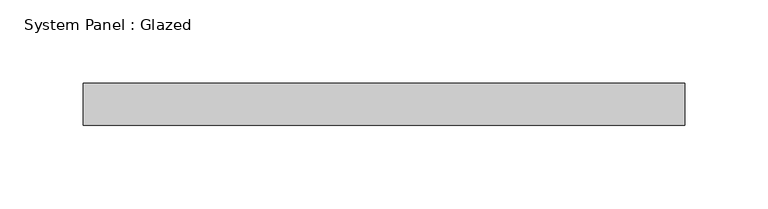
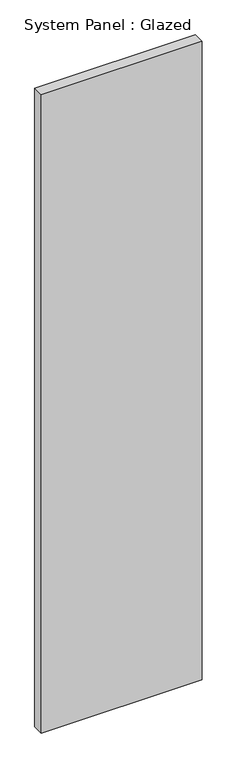
"""IFC4 building model written with IfcOpenShell, lengths in millimetres: plate geometry, System Panel : Glazed."""

from ifc_helpers import new_model, si_unit, origin, origin_with_axes, place, context, project, spatial, polyline, outline, extrude, source, transform, mapped, element, save


def system_panel_glazed_1aec69dd(model_context):
    return source(origin(), model_context, "Body", "SweptSolid", [
        extrude(outline(polyline([(180.975, 19.05), (-180.975, 19.05), (-180.975, 44.45), (180.975, 44.45), (180.975, 19.05)])), origin_with_axes(), (0.0, 0.0, 1.0), 1519.9538703),
    ])


if __name__ == "__main__":
    model = new_model("IFC4")
    model_context = context("Model", 3, world=origin())
    ifc_project = project(units=[si_unit("LENGTHUNIT", "METRE", prefix="MILLI")], contexts=[model_context])
    site = spatial("IfcSite", under=ifc_project)
    building = spatial("IfcBuilding", under=site)
    placement = place(None, origin())
    system_panel_glazed_shape = system_panel_glazed_1aec69dd(model_context)
    element("IfcPlate", 1, ObjectType="System Panel : Glazed", at=placement, inside=building, context=model_context, shape_type="MappedRepresentation", body=[
        mapped(system_panel_glazed_shape, transform((0.0, 0.0, 0.0), x_axis=(1.0, 0.0, 0.0), y_axis=(0.0, 1.0, 0.0), z_axis=(0.0, 0.0, 1.0))),
    ])
    save(model, "model.ifc")

# Revit data of these elements
# Type "System Panel : Glazed"
#   Construction Type Id = "GSP4R"
#   Analytic Construction = "1/8 in Pilkington single glazing"
#   Visual Light Transmittance = 0.9
#   Solar Heat Gain Coefficient = 0.86
#   Heat Transfer Coefficient (U) = 1.18115 BTU/(h·ft²·°F)
#   Define Thermal Properties by = 1
# Element 1 (IfcPlate, "System Panel : Glazed")
#   Materials on its faces: "Glass"
# Materials
#   "Glass": class "Glass", colour RGB 0 128 192, transparency 0.75, Description = "Soda Lime Glass", Cost = 0
